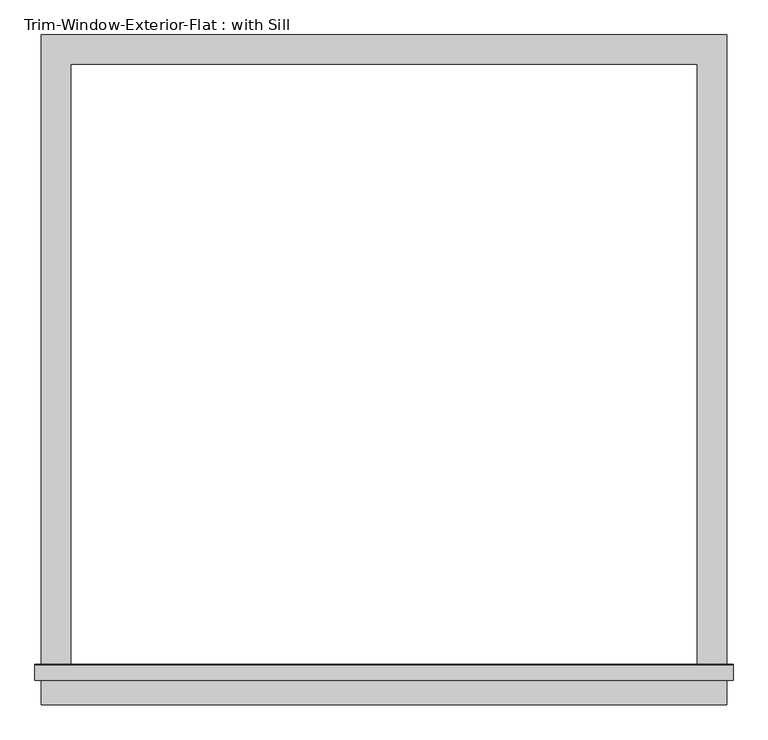
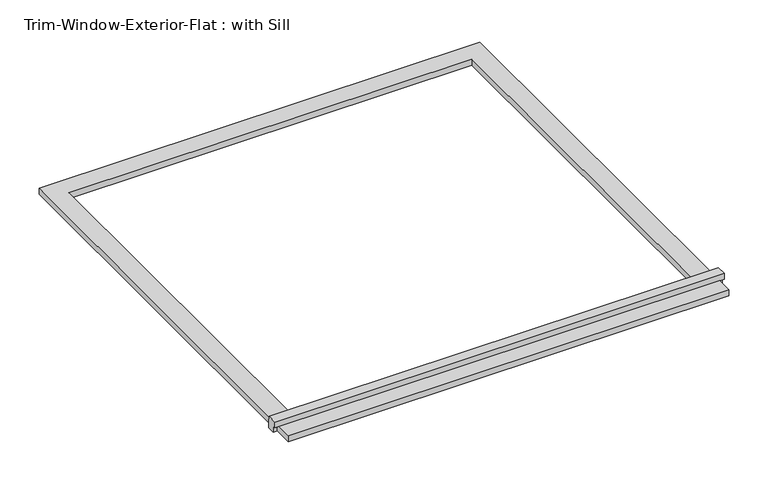
"""IFC4 building model written with IfcOpenShell, lengths in millimetres: proxy geometry, Trim-Window-Exterior-Flat : with Sill."""

from ifc_helpers import new_model, si_unit, frame, origin, origin_with_axes, place, context, project, spatial, polyline, outline, extrude, source, transform, mapped, element, save


def trim_window_exterior_flat_with_sill_91d32942(model_context):
    return source(origin(), model_context, "Body", "SweptSolid", [
        extrude(outline(polyline([(666.75, -1190.5823709), (666.75, -1247.7323709), (-666.75, -1247.7323709), (-666.75, -1190.5823709), (666.75, -1190.5823709)])), origin_with_axes(), (0.0, 0.0, 1.0), 19.05),
        extrude(outline(polyline([(-1200.15, 38.1), (-1170.8580645, 38.1), (-1168.4, 19.05), (-1168.4, 0.0), (-1190.5823709, 0.0), (-1190.5823709, 19.05), (-1200.15, 19.05), (-1200.15, 38.1)])), frame((-679.45, 0.0, 0.0), z_axis=(1.0, 0.0, 0.0), x_axis=(0.0, 1.0, 0.0)), (0.0, 0.0, 1.0), 1358.9),
        extrude(outline(polyline([(-666.75, 57.15), (666.75, 57.15), (666.75, -1168.4), (609.6, -1168.4), (609.6, 0.0), (-609.6, 0.0), (-609.6, -1168.4), (-666.75, -1168.4), (-666.75, 57.15)])), origin_with_axes(), (0.0, 0.0, 1.0), 19.05),
    ])


if __name__ == "__main__":
    model = new_model("IFC4")
    model_context = context("Model", 3, world=origin())
    ifc_project = project(units=[si_unit("LENGTHUNIT", "METRE", prefix="MILLI")], contexts=[model_context])
    site = spatial("IfcSite", under=ifc_project)
    building = spatial("IfcBuilding", under=site)
    placement = place(None, origin())
    trim_window_exterior_flat_with_sill_shape = trim_window_exterior_flat_with_sill_91d32942(model_context)
    element("IfcBuildingElementProxy", 1, Name="Trim-Window-Exterior-Flat : with Sill", ObjectType="Trim-Window-Exterior-Flat : with Sill", at=placement, inside=building, context=model_context, shape_type="MappedRepresentation", body=[
        mapped(trim_window_exterior_flat_with_sill_shape, transform((0.0, 0.0, 0.0), x_axis=(1.0, 0.0, 0.0), y_axis=(0.0, 1.0, 0.0), z_axis=(0.0, 0.0, 1.0))),
    ])
    save(model, "model.ifc")

# Revit data of these elements
# Type "Trim-Window-Exterior-Flat : with Sill"
#   Trim Width = 0' - 2 1/4"
#   Trim Thickness_Picture Frame = 0' - 1 1/4"
#   Trim Thickness_with Sill = 0' - 0 3/4"
#   Sill Thickness = 0' - 1 1/4"
#   Opening Width [instance default] = 2' - 0"
#   Opening Height [instance default] = 3' - 0"
#   Default Elevation = 4' - 0"
#   Sill = yes
#   Picture Frame = no
#   Trim Material [instance default] = none
# Element 1 (IfcBuildingElementProxy, "Trim-Window-Exterior-Flat : with Sill")
#   Opening Width = 4' - 0"
#   Opening Height = 3' - 10"
#   Trim Material = Clad - White
#   Materials on its faces: "Clad - White"
# Materials
#   "Clad - White": class "Wood", colour RGB 242 242 238, transparency 0, Cost = 0
